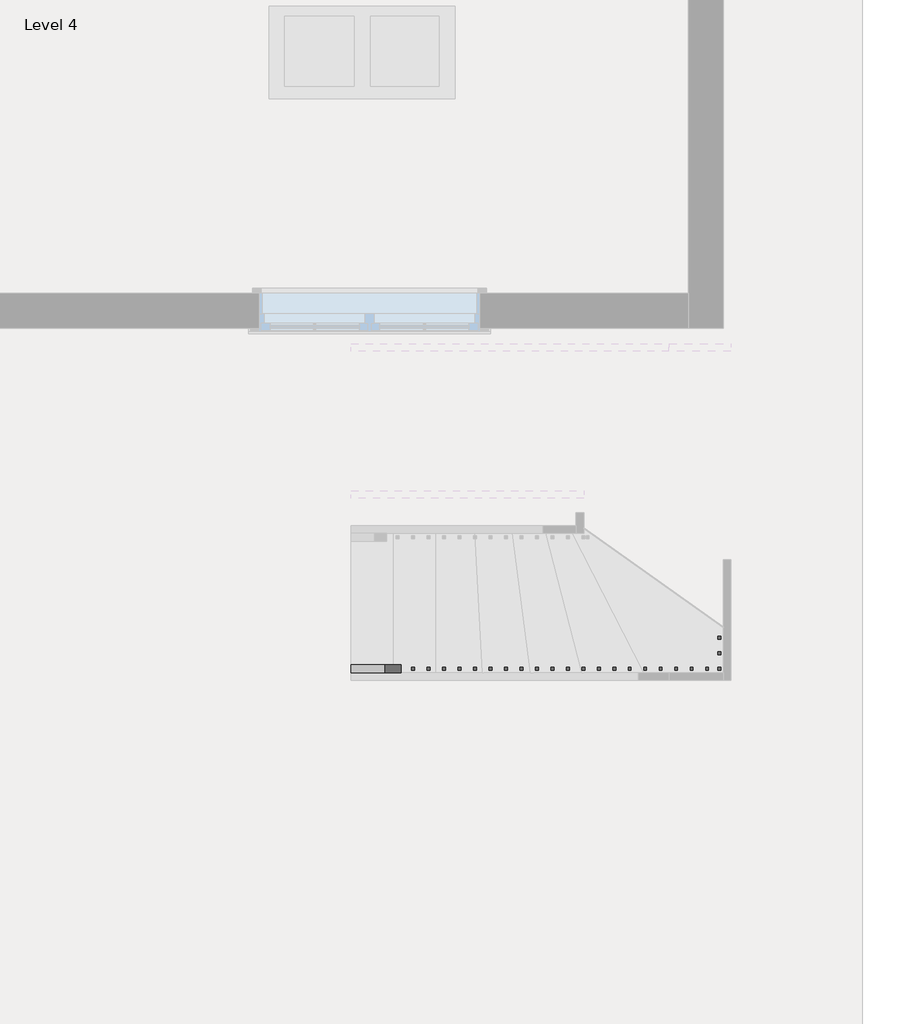
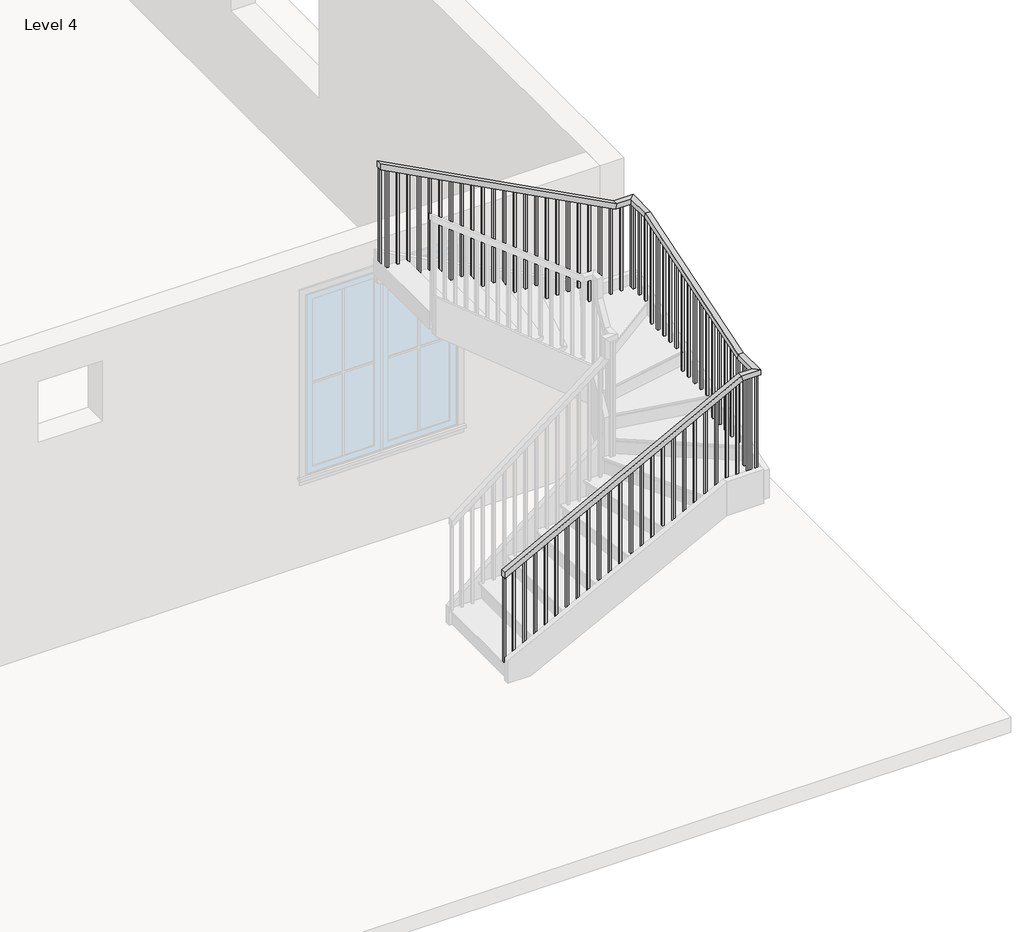
# One storey, part 2 of 3: 1 railing.
"""IFC4 building model written with IfcOpenShell, lengths in millimetres."""

from ifc_helpers import new_model, si_unit, frame, origin, place, context, project, spatial, polyline, outline, extrude, faceted_brep, element, save

model = new_model("IFC4")

# Units and contexts
model_context = context("Model", 3, world=origin())
ifc_project = project(units=[si_unit("LENGTHUNIT", "METRE", prefix="MILLI")], contexts=[model_context])

# Site, building, storey
site = spatial("IfcSite", under=ifc_project)
building = spatial("IfcBuilding", under=site)
storey = spatial("IfcBuildingStorey", under=building, Name="Level 4", Elevation=6400.8)

# Railing
placement = place(None, origin())
element("IfcRailing", 1, ObjectType="Handrail - Rectangular", at=placement, inside=storey, context=model_context, shape_type="SolidModel", body=[
    faceted_brep([(531.7538115, -7514.4090409, 7484.5333333), (531.7538115, -7514.4090409, 7427.0742652), (531.7538115, -7565.2090409, 7427.0742652), (531.7538115, -7565.2090409, 7484.5333333), (2789.4788736, -7514.4090409, 8677.8239201), (2802.0779381, -7514.4090409, 8627.0239201), (2802.0779381, -7565.2090409, 8627.0239201), (2789.4788736, -7565.2090409, 8677.8239201), (2923.0855034, -7269.9465826, 8627.0239201), (2923.0855034, -7277.8971587, 8677.8239201), (2923.0855034, -5744.320923, 9169.9094132), (2923.0855034, -5736.3703469, 9119.1094132), (2973.8855034, -7269.9465826, 8627.0239201), (2973.8855034, -5736.3703469, 9119.1094132), (2973.8855034, -7277.8971587, 8677.8239201), (2973.8855034, -5744.320923, 9169.9094132), (531.7538115, -5507.8090409, 10363.2), (531.7538115, -5457.0090409, 10363.2), (531.7538115, -5457.0090409, 10305.7409318), (531.7538115, -5507.8090409, 10305.7409318), (2776.879809, -5507.8090409, 9119.1094132), (2789.4788736, -5507.8090409, 9169.9094132), (2776.879809, -5457.0090409, 9119.1094132), (2789.4788736, -5457.0090409, 9169.9094132), (2923.0855034, -7514.4090409, 8677.8239201), (2923.0855034, -7514.4090409, 8627.0239201), (2973.8855034, -7565.2090409, 8627.0239201), (2973.8855034, -7565.2090409, 8677.8239201), (2923.0855034, -5507.8090409, 9169.9094132), (2923.0855034, -5507.8090409, 9119.1094132), (2973.8855034, -5457.0090409, 9119.1094132), (2973.8855034, -5457.0090409, 9169.9094132)], [[[0, 1, 2, 3]], [[1, 0, 4, 5]], [[2, 1, 5, 6]], [[3, 2, 6, 7]], [[0, 3, 7, 4]], [[8, 9, 10, 11]], [[12, 8, 11, 13]], [[14, 12, 13, 15]], [[9, 14, 15, 10]], [[16, 17, 18, 19]], [[20, 21, 16, 19]], [[22, 20, 19, 18]], [[23, 22, 18, 17]], [[21, 23, 17, 16]], [[5, 4, 24, 25]], [[6, 5, 25, 26]], [[7, 6, 26, 27]], [[4, 7, 27, 24]], [[25, 24, 9, 8]], [[26, 25, 8, 12]], [[27, 26, 12, 14]], [[24, 27, 14, 9]], [[11, 10, 28, 29]], [[13, 11, 29, 30]], [[15, 13, 30, 31]], [[10, 15, 31, 28]], [[29, 28, 21, 20]], [[30, 29, 20, 22]], [[31, 30, 22, 23]], [[28, 31, 23, 21]]]),
    extrude(outline(polyline([(10258.4597858, 621.2105034), (10268.5284102, 602.1605034), (9279.4666667, 602.1605034), (9279.4666667, 621.2105034), (10258.4597858, 621.2105034)])), frame((0.0, -5491.9340409, 0.0), z_axis=(0.0, 1.0, 0.0), x_axis=(0.0, 0.0, 1.0)), (0.0, 0.0, 1.0), 19.05),
    extrude(outline(polyline([(10204.7604556, 722.8105034), (10214.82908, 703.7605034), (9279.4666667, 703.7605034), (9279.4666667, 722.8105034), (10204.7604556, 722.8105034)])), frame((0.0, -5491.9340409, 0.0), z_axis=(0.0, 1.0, 0.0), x_axis=(0.0, 0.0, 1.0)), (0.0, 0.0, 1.0), 19.05),
    extrude(outline(polyline([(10151.0611254, 824.4105034), (10161.1297498, 805.3605034), (9110.1333333, 805.3605034), (9110.1333333, 824.4105034), (10151.0611254, 824.4105034)])), frame((0.0, -5491.9340409, 0.0), z_axis=(0.0, 1.0, 0.0), x_axis=(0.0, 0.0, 1.0)), (0.0, 0.0, 1.0), 19.05),
    extrude(outline(polyline([(10097.3617952, 926.0105034), (10107.4304196, 906.9605034), (9110.1333333, 906.9605034), (9110.1333333, 926.0105034), (10097.3617952, 926.0105034)])), frame((0.0, -5491.9340409, 0.0), z_axis=(0.0, 1.0, 0.0), x_axis=(0.0, 0.0, 1.0)), (0.0, 0.0, 1.0), 19.05),
    extrude(outline(polyline([(10043.662465, 1027.6105034), (10053.7310894, 1008.5605034), (9110.1333333, 1008.5605034), (9110.1333333, 1027.6105034), (10043.662465, 1027.6105034)])), frame((0.0, -5491.9340409, 0.0), z_axis=(0.0, 1.0, 0.0), x_axis=(0.0, 0.0, 1.0)), (0.0, 0.0, 1.0), 19.05),
    extrude(outline(polyline([(9989.9631348, 1129.2105034), (10000.0317592, 1110.1605034), (8940.8, 1110.1605034), (8940.8, 1129.2105034), (9989.9631348, 1129.2105034)])), frame((0.0, -5491.9340409, 0.0), z_axis=(0.0, 1.0, 0.0), x_axis=(0.0, 0.0, 1.0)), (0.0, 0.0, 1.0), 19.05),
    extrude(outline(polyline([(9936.2638046, 1230.8105034), (9946.332429, 1211.7605034), (8940.8, 1211.7605034), (8940.8, 1230.8105034), (9936.2638046, 1230.8105034)])), frame((0.0, -5491.9340409, 0.0), z_axis=(0.0, 1.0, 0.0), x_axis=(0.0, 0.0, 1.0)), (0.0, 0.0, 1.0), 19.05),
    extrude(outline(polyline([(9882.5644744, 1332.4105034), (9892.6330988, 1313.3605034), (8940.8, 1313.3605034), (8940.8, 1332.4105034), (9882.5644744, 1332.4105034)])), frame((0.0, -5491.9340409, 0.0), z_axis=(0.0, 1.0, 0.0), x_axis=(0.0, 0.0, 1.0)), (0.0, 0.0, 1.0), 19.05),
    extrude(outline(polyline([(9828.8651442, 1434.0105034), (9838.9337686, 1414.9605034), (8771.4666667, 1414.9605034), (8771.4666667, 1434.0105034), (9828.8651442, 1434.0105034)])), frame((0.0, -5491.9340409, 0.0), z_axis=(0.0, 1.0, 0.0), x_axis=(0.0, 0.0, 1.0)), (0.0, 0.0, 1.0), 19.05),
    extrude(outline(polyline([(9775.165814, 1535.6105034), (9785.2344384, 1516.5605034), (8771.4666667, 1516.5605034), (8771.4666667, 1535.6105034), (9775.165814, 1535.6105034)])), frame((0.0, -5491.9340409, 0.0), z_axis=(0.0, 1.0, 0.0), x_axis=(0.0, 0.0, 1.0)), (0.0, 0.0, 1.0), 19.05),
    extrude(outline(polyline([(9721.4664838, 1637.2105034), (9731.5351082, 1618.1605034), (8771.4666667, 1618.1605034), (8771.4666667, 1637.2105034), (9721.4664838, 1637.2105034)])), frame((0.0, -5491.9340409, 0.0), z_axis=(0.0, 1.0, 0.0), x_axis=(0.0, 0.0, 1.0)), (0.0, 0.0, 1.0), 19.05),
    extrude(outline(polyline([(9667.7671536, 1738.8105034), (9677.835778, 1719.7605034), (8602.1333333, 1719.7605034), (8602.1333333, 1738.8105034), (9667.7671536, 1738.8105034)])), frame((0.0, -5491.9340409, 0.0), z_axis=(0.0, 1.0, 0.0), x_axis=(0.0, 0.0, 1.0)), (0.0, 0.0, 1.0), 19.05),
    extrude(outline(polyline([(9614.0678234, 1840.4105034), (9624.1364478, 1821.3605034), (8602.1333333, 1821.3605034), (8602.1333333, 1840.4105034), (9614.0678234, 1840.4105034)])), frame((0.0, -5491.9340409, 0.0), z_axis=(0.0, 1.0, 0.0), x_axis=(0.0, 0.0, 1.0)), (0.0, 0.0, 1.0), 19.05),
    extrude(outline(polyline([(9560.3684932, 1942.0105034), (9570.4371176, 1922.9605034), (8602.1333333, 1922.9605034), (8602.1333333, 1942.0105034), (9560.3684932, 1942.0105034)])), frame((0.0, -5491.9340409, 0.0), z_axis=(0.0, 1.0, 0.0), x_axis=(0.0, 0.0, 1.0)), (0.0, 0.0, 1.0), 19.05),
    extrude(outline(polyline([(9506.669163, 2043.6105034), (9516.7377874, 2024.5605034), (8602.1333333, 2024.5605034), (8602.1333333, 2043.6105034), (9506.669163, 2043.6105034)])), frame((0.0, -5491.9340409, 0.0), z_axis=(0.0, 1.0, 0.0), x_axis=(0.0, 0.0, 1.0)), (0.0, 0.0, 1.0), 19.05),
    extrude(outline(polyline([(9452.9698328, 2145.2105034), (9463.0384572, 2126.1605034), (8432.8, 2126.1605034), (8432.8, 2145.2105034), (9452.9698328, 2145.2105034)])), frame((0.0, -5491.9340409, 0.0), z_axis=(0.0, 1.0, 0.0), x_axis=(0.0, 0.0, 1.0)), (0.0, 0.0, 1.0), 19.05),
    extrude(outline(polyline([(9399.2705026, 2246.8105034), (9409.339127, 2227.7605034), (8432.8, 2227.7605034), (8432.8, 2246.8105034), (9399.2705026, 2246.8105034)])), frame((0.0, -5491.9340409, 0.0), z_axis=(0.0, 1.0, 0.0), x_axis=(0.0, 0.0, 1.0)), (0.0, 0.0, 1.0), 19.05),
    extrude(outline(polyline([(9345.5711724, 2348.4105034), (9355.6397968, 2329.3605034), (8432.8, 2329.3605034), (8432.8, 2348.4105034), (9345.5711724, 2348.4105034)])), frame((0.0, -5491.9340409, 0.0), z_axis=(0.0, 1.0, 0.0), x_axis=(0.0, 0.0, 1.0)), (0.0, 0.0, 1.0), 19.05),
    extrude(outline(polyline([(9291.8718422, 2450.0105034), (9301.9404666, 2430.9605034), (8432.8, 2430.9605034), (8432.8, 2450.0105034), (9291.8718422, 2450.0105034)])), frame((0.0, -5491.9340409, 0.0), z_axis=(0.0, 1.0, 0.0), x_axis=(0.0, 0.0, 1.0)), (0.0, 0.0, 1.0), 19.05),
    extrude(outline(polyline([(9238.172512, 2551.6105034), (9248.2411364, 2532.5605034), (8263.4666667, 2532.5605034), (8263.4666667, 2551.6105034), (9238.172512, 2551.6105034)])), frame((0.0, -5491.9340409, 0.0), z_axis=(0.0, 1.0, 0.0), x_axis=(0.0, 0.0, 1.0)), (0.0, 0.0, 1.0), 19.05),
    extrude(outline(polyline([(9184.4731818, 2653.2105034), (9194.5418062, 2634.1605034), (8263.4666667, 2634.1605034), (8263.4666667, 2653.2105034), (9184.4731818, 2653.2105034)])), frame((0.0, -5491.9340409, 0.0), z_axis=(0.0, 1.0, 0.0), x_axis=(0.0, 0.0, 1.0)), (0.0, 0.0, 1.0), 19.05),
    extrude(outline(polyline([(9130.7738516, 2754.8105034), (9140.842476, 2735.7605034), (8263.4666667, 2735.7605034), (8263.4666667, 2754.8105034), (9130.7738516, 2754.8105034)])), frame((0.0, -5491.9340409, 0.0), z_axis=(0.0, 1.0, 0.0), x_axis=(0.0, 0.0, 1.0)), (0.0, 0.0, 1.0), 19.05),
    extrude(outline(polyline([(2856.4105034, -5472.8840409), (2856.4105034, -5491.9340409), (2837.3605034, -5491.9340409), (2837.3605034, -5472.8840409), (2856.4105034, -5472.8840409)])), frame((0.0, 0.0, 8263.4666667), z_axis=(0.0, 0.0, 1.0), x_axis=(1.0, 0.0, 0.0)), (0.0, 0.0, 1.0), 855.6427466),
    extrude(outline(polyline([(2958.0105034, -5517.3340409), (2938.9605034, -5517.3340409), (2938.9605034, -5498.2840409), (2958.0105034, -5498.2840409), (2958.0105034, -5517.3340409)])), frame((0.0, 0.0, 8263.4666667), z_axis=(0.0, 0.0, 1.0), x_axis=(1.0, 0.0, 0.0)), (0.0, 0.0, 1.0), 855.6427466),
    extrude(outline(polyline([(2958.0105034, -5618.9340409), (2938.9605034, -5618.9340409), (2938.9605034, -5599.8840409), (2958.0105034, -5599.8840409), (2958.0105034, -5618.9340409)])), frame((0.0, 0.0, 8263.4666667), z_axis=(0.0, 0.0, 1.0), x_axis=(1.0, 0.0, 0.0)), (0.0, 0.0, 1.0), 855.6427466),
    extrude(outline(polyline([(2958.0105034, -5720.5340409), (2938.9605034, -5720.5340409), (2938.9605034, -5701.4840409), (2958.0105034, -5701.4840409), (2958.0105034, -5720.5340409)])), frame((0.0, 0.0, 8263.4666667), z_axis=(0.0, 0.0, 1.0), x_axis=(1.0, 0.0, 0.0)), (0.0, 0.0, 1.0), 855.6427466),
    extrude(outline(polyline([(-5822.1340409, 9091.5900316), (-5803.0840409, 9097.7026907), (-5803.0840409, 8094.1333333), (-5822.1340409, 8094.1333333), (-5822.1340409, 9091.5900316)])), frame((2938.9605034, 0.0, 0.0), z_axis=(1.0, 0.0, 0.0), x_axis=(0.0, 1.0, 0.0)), (0.0, 0.0, 1.0), 19.05),
    extrude(outline(polyline([(-5923.7340409, 9058.9891834), (-5904.6840409, 9065.1018425), (-5904.6840409, 8094.1333333), (-5923.7340409, 8094.1333333), (-5923.7340409, 9058.9891834)])), frame((2938.9605034, 0.0, 0.0), z_axis=(1.0, 0.0, 0.0), x_axis=(0.0, 1.0, 0.0)), (0.0, 0.0, 1.0), 19.05),
    extrude(outline(polyline([(-6025.3340409, 9026.3883352), (-6006.2840409, 9032.5009942), (-6006.2840409, 8094.1333333), (-6025.3340409, 8094.1333333), (-6025.3340409, 9026.3883352)])), frame((2938.9605034, 0.0, 0.0), z_axis=(1.0, 0.0, 0.0), x_axis=(0.0, 1.0, 0.0)), (0.0, 0.0, 1.0), 19.05),
    extrude(outline(polyline([(-6126.9340409, 8993.787487), (-6107.8840409, 8999.900146), (-6107.8840409, 8094.1333333), (-6126.9340409, 8094.1333333), (-6126.9340409, 8993.787487)])), frame((2938.9605034, 0.0, 0.0), z_axis=(1.0, 0.0, 0.0), x_axis=(0.0, 1.0, 0.0)), (0.0, 0.0, 1.0), 19.05),
    extrude(outline(polyline([(-6228.5340409, 8961.1866387), (-6209.4840409, 8967.2992978), (-6209.4840409, 8094.1333333), (-6228.5340409, 8094.1333333), (-6228.5340409, 8961.1866387)])), frame((2938.9605034, 0.0, 0.0), z_axis=(1.0, 0.0, 0.0), x_axis=(0.0, 1.0, 0.0)), (0.0, 0.0, 1.0), 19.05),
    extrude(outline(polyline([(-6330.1340409, 8928.5857905), (-6311.0840409, 8934.6984495), (-6311.0840409, 7924.8), (-6330.1340409, 7924.8), (-6330.1340409, 8928.5857905)])), frame((2938.9605034, 0.0, 0.0), z_axis=(1.0, 0.0, 0.0), x_axis=(0.0, 1.0, 0.0)), (0.0, 0.0, 1.0), 19.05),
    extrude(outline(polyline([(-6431.7340409, 8895.9849423), (-6412.6840409, 8902.0976013), (-6412.6840409, 7924.8), (-6431.7340409, 7924.8), (-6431.7340409, 8895.9849423)])), frame((2938.9605034, 0.0, 0.0), z_axis=(1.0, 0.0, 0.0), x_axis=(0.0, 1.0, 0.0)), (0.0, 0.0, 1.0), 19.05),
    extrude(outline(polyline([(-6533.3340409, 8863.384094), (-6514.2840409, 8869.4967531), (-6514.2840409, 7924.8), (-6533.3340409, 7924.8), (-6533.3340409, 8863.384094)])), frame((2938.9605034, 0.0, 0.0), z_axis=(1.0, 0.0, 0.0), x_axis=(0.0, 1.0, 0.0)), (0.0, 0.0, 1.0), 19.05),
    extrude(outline(polyline([(-6634.9340409, 8830.7832458), (-6615.8840409, 8836.8959049), (-6615.8840409, 7924.8), (-6634.9340409, 7924.8), (-6634.9340409, 8830.7832458)])), frame((2938.9605034, 0.0, 0.0), z_axis=(1.0, 0.0, 0.0), x_axis=(0.0, 1.0, 0.0)), (0.0, 0.0, 1.0), 19.05),
    extrude(outline(polyline([(-6736.5340409, 8798.1823976), (-6717.4840409, 8804.2950566), (-6717.4840409, 7924.8), (-6736.5340409, 7924.8), (-6736.5340409, 8798.1823976)])), frame((2938.9605034, 0.0, 0.0), z_axis=(1.0, 0.0, 0.0), x_axis=(0.0, 1.0, 0.0)), (0.0, 0.0, 1.0), 19.05),
    extrude(outline(polyline([(-6838.1340409, 8765.5815494), (-6819.0840409, 8771.6942084), (-6819.0840409, 7755.4666667), (-6838.1340409, 7755.4666667), (-6838.1340409, 8765.5815494)])), frame((2938.9605034, 0.0, 0.0), z_axis=(1.0, 0.0, 0.0), x_axis=(0.0, 1.0, 0.0)), (0.0, 0.0, 1.0), 19.05),
    extrude(outline(polyline([(-6939.7340409, 8732.9807011), (-6920.6840409, 8739.0933602), (-6920.6840409, 7755.4666667), (-6939.7340409, 7755.4666667), (-6939.7340409, 8732.9807011)])), frame((2938.9605034, 0.0, 0.0), z_axis=(1.0, 0.0, 0.0), x_axis=(0.0, 1.0, 0.0)), (0.0, 0.0, 1.0), 19.05),
    extrude(outline(polyline([(-7041.3340409, 8700.3798529), (-7022.2840409, 8706.492512), (-7022.2840409, 7755.4666667), (-7041.3340409, 7755.4666667), (-7041.3340409, 8700.3798529)])), frame((2938.9605034, 0.0, 0.0), z_axis=(1.0, 0.0, 0.0), x_axis=(0.0, 1.0, 0.0)), (0.0, 0.0, 1.0), 19.05),
    extrude(outline(polyline([(-7142.9340409, 8667.7790047), (-7123.8840409, 8673.8916637), (-7123.8840409, 7755.4666667), (-7142.9340409, 7755.4666667), (-7142.9340409, 8667.7790047)])), frame((2938.9605034, 0.0, 0.0), z_axis=(1.0, 0.0, 0.0), x_axis=(0.0, 1.0, 0.0)), (0.0, 0.0, 1.0), 19.05),
    extrude(outline(polyline([(-7244.5340409, 8635.1781565), (-7225.4840409, 8641.2908155), (-7225.4840409, 7755.4666667), (-7244.5340409, 7755.4666667), (-7244.5340409, 8635.1781565)])), frame((2938.9605034, 0.0, 0.0), z_axis=(1.0, 0.0, 0.0), x_axis=(0.0, 1.0, 0.0)), (0.0, 0.0, 1.0), 19.05),
    extrude(outline(polyline([(2958.0105034, -7346.1340409), (2938.9605034, -7346.1340409), (2938.9605034, -7327.0840409), (2958.0105034, -7327.0840409), (2958.0105034, -7346.1340409)])), frame((0.0, 0.0, 7586.1333333), z_axis=(0.0, 0.0, 1.0), x_axis=(1.0, 0.0, 0.0)), (0.0, 0.0, 1.0), 1040.8905868),
    extrude(outline(polyline([(2958.0105034, -7447.7340409), (2938.9605034, -7447.7340409), (2938.9605034, -7428.6840409), (2958.0105034, -7428.6840409), (2958.0105034, -7447.7340409)])), frame((0.0, 0.0, 7586.1333333), z_axis=(0.0, 0.0, 1.0), x_axis=(1.0, 0.0, 0.0)), (0.0, 0.0, 1.0), 1040.8905868),
    extrude(outline(polyline([(2859.0288115, -7549.3340409), (2859.0288115, -7530.2840409), (2878.0788115, -7530.2840409), (2878.0788115, -7549.3340409), (2859.0288115, -7549.3340409)])), frame((0.0, 0.0, 7586.1333333), z_axis=(0.0, 0.0, 1.0), x_axis=(1.0, 0.0, 0.0)), (0.0, 0.0, 1.0), 1040.8905868),
    extrude(outline(polyline([(8613.4938418, 2776.4788115), (8603.4252174, 2757.4288115), (7586.1333333, 2757.4288115), (7586.1333333, 2776.4788115), (8613.4938418, 2776.4788115)])), frame((0.0, -7549.3340409, 0.0), z_axis=(0.0, 1.0, 0.0), x_axis=(0.0, 0.0, 1.0)), (0.0, 0.0, 1.0), 19.05),
    extrude(outline(polyline([(8559.7945116, 2674.8788115), (8549.7258872, 2655.8288115), (7586.1333333, 2655.8288115), (7586.1333333, 2674.8788115), (8559.7945116, 2674.8788115)])), frame((0.0, -7549.3340409, 0.0), z_axis=(0.0, 1.0, 0.0), x_axis=(0.0, 0.0, 1.0)), (0.0, 0.0, 1.0), 19.05),
    extrude(outline(polyline([(8506.0951814, 2573.2788115), (8496.026557, 2554.2288115), (7586.1333333, 2554.2288115), (7586.1333333, 2573.2788115), (8506.0951814, 2573.2788115)])), frame((0.0, -7549.3340409, 0.0), z_axis=(0.0, 1.0, 0.0), x_axis=(0.0, 0.0, 1.0)), (0.0, 0.0, 1.0), 19.05),
    extrude(outline(polyline([(8452.3958512, 2471.6788115), (8442.3272268, 2452.6288115), (7586.1333333, 2452.6288115), (7586.1333333, 2471.6788115), (8452.3958512, 2471.6788115)])), frame((0.0, -7549.3340409, 0.0), z_axis=(0.0, 1.0, 0.0), x_axis=(0.0, 0.0, 1.0)), (0.0, 0.0, 1.0), 19.05),
    extrude(outline(polyline([(8398.696521, 2370.0788115), (8388.6278966, 2351.0288115), (7416.8, 2351.0288115), (7416.8, 2370.0788115), (8398.696521, 2370.0788115)])), frame((0.0, -7549.3340409, 0.0), z_axis=(0.0, 1.0, 0.0), x_axis=(0.0, 0.0, 1.0)), (0.0, 0.0, 1.0), 19.05),
    extrude(outline(polyline([(8344.9971908, 2268.4788115), (8334.9285664, 2249.4288115), (7416.8, 2249.4288115), (7416.8, 2268.4788115), (8344.9971908, 2268.4788115)])), frame((0.0, -7549.3340409, 0.0), z_axis=(0.0, 1.0, 0.0), x_axis=(0.0, 0.0, 1.0)), (0.0, 0.0, 1.0), 19.05),
    extrude(outline(polyline([(8291.2978606, 2166.8788115), (8281.2292362, 2147.8288115), (7416.8, 2147.8288115), (7416.8, 2166.8788115), (8291.2978606, 2166.8788115)])), frame((0.0, -7549.3340409, 0.0), z_axis=(0.0, 1.0, 0.0), x_axis=(0.0, 0.0, 1.0)), (0.0, 0.0, 1.0), 19.05),
    extrude(outline(polyline([(8237.5985304, 2065.2788115), (8227.529906, 2046.2288115), (7416.8, 2046.2288115), (7416.8, 2065.2788115), (8237.5985304, 2065.2788115)])), frame((0.0, -7549.3340409, 0.0), z_axis=(0.0, 1.0, 0.0), x_axis=(0.0, 0.0, 1.0)), (0.0, 0.0, 1.0), 19.05),
    extrude(outline(polyline([(8183.8992002, 1963.6788115), (8173.8305758, 1944.6288115), (7247.4666667, 1944.6288115), (7247.4666667, 1963.6788115), (8183.8992002, 1963.6788115)])), frame((0.0, -7549.3340409, 0.0), z_axis=(0.0, 1.0, 0.0), x_axis=(0.0, 0.0, 1.0)), (0.0, 0.0, 1.0), 19.05),
    extrude(outline(polyline([(8130.19987, 1862.0788115), (8120.1312456, 1843.0288115), (7247.4666667, 1843.0288115), (7247.4666667, 1862.0788115), (8130.19987, 1862.0788115)])), frame((0.0, -7549.3340409, 0.0), z_axis=(0.0, 1.0, 0.0), x_axis=(0.0, 0.0, 1.0)), (0.0, 0.0, 1.0), 19.05),
    extrude(outline(polyline([(8076.5005398, 1760.4788115), (8066.4319154, 1741.4288115), (7247.4666667, 1741.4288115), (7247.4666667, 1760.4788115), (8076.5005398, 1760.4788115)])), frame((0.0, -7549.3340409, 0.0), z_axis=(0.0, 1.0, 0.0), x_axis=(0.0, 0.0, 1.0)), (0.0, 0.0, 1.0), 19.05),
    extrude(outline(polyline([(8022.8012096, 1658.8788115), (8012.7325852, 1639.8288115), (7078.1333333, 1639.8288115), (7078.1333333, 1658.8788115), (8022.8012096, 1658.8788115)])), frame((0.0, -7549.3340409, 0.0), z_axis=(0.0, 1.0, 0.0), x_axis=(0.0, 0.0, 1.0)), (0.0, 0.0, 1.0), 19.05),
    extrude(outline(polyline([(7969.1018794, 1557.2788115), (7959.033255, 1538.2288115), (7078.1333333, 1538.2288115), (7078.1333333, 1557.2788115), (7969.1018794, 1557.2788115)])), frame((0.0, -7549.3340409, 0.0), z_axis=(0.0, 1.0, 0.0), x_axis=(0.0, 0.0, 1.0)), (0.0, 0.0, 1.0), 19.05),
    extrude(outline(polyline([(7915.4025492, 1455.6788115), (7905.3339248, 1436.6288115), (7078.1333333, 1436.6288115), (7078.1333333, 1455.6788115), (7915.4025492, 1455.6788115)])), frame((0.0, -7549.3340409, 0.0), z_axis=(0.0, 1.0, 0.0), x_axis=(0.0, 0.0, 1.0)), (0.0, 0.0, 1.0), 19.05),
    extrude(outline(polyline([(7861.703219, 1354.0788115), (7851.6345946, 1335.0288115), (6908.8, 1335.0288115), (6908.8, 1354.0788115), (7861.703219, 1354.0788115)])), frame((0.0, -7549.3340409, 0.0), z_axis=(0.0, 1.0, 0.0), x_axis=(0.0, 0.0, 1.0)), (0.0, 0.0, 1.0), 19.05),
    extrude(outline(polyline([(7808.0038888, 1252.4788115), (7797.9352644, 1233.4288115), (6908.8, 1233.4288115), (6908.8, 1252.4788115), (7808.0038888, 1252.4788115)])), frame((0.0, -7549.3340409, 0.0), z_axis=(0.0, 1.0, 0.0), x_axis=(0.0, 0.0, 1.0)), (0.0, 0.0, 1.0), 19.05),
    extrude(outline(polyline([(7754.3045586, 1150.8788115), (7744.2359342, 1131.8288115), (6908.8, 1131.8288115), (6908.8, 1150.8788115), (7754.3045586, 1150.8788115)])), frame((0.0, -7549.3340409, 0.0), z_axis=(0.0, 1.0, 0.0), x_axis=(0.0, 0.0, 1.0)), (0.0, 0.0, 1.0), 19.05),
    extrude(outline(polyline([(7700.6052284, 1049.2788115), (7690.536604, 1030.2288115), (6739.4666667, 1030.2288115), (6739.4666667, 1049.2788115), (7700.6052284, 1049.2788115)])), frame((0.0, -7549.3340409, 0.0), z_axis=(0.0, 1.0, 0.0), x_axis=(0.0, 0.0, 1.0)), (0.0, 0.0, 1.0), 19.05),
    extrude(outline(polyline([(7646.9058982, 947.6788115), (7636.8372738, 928.6288115), (6739.4666667, 928.6288115), (6739.4666667, 947.6788115), (7646.9058982, 947.6788115)])), frame((0.0, -7549.3340409, 0.0), z_axis=(0.0, 1.0, 0.0), x_axis=(0.0, 0.0, 1.0)), (0.0, 0.0, 1.0), 19.05),
    extrude(outline(polyline([(7593.206568, 846.0788115), (7583.1379436, 827.0288115), (6739.4666667, 827.0288115), (6739.4666667, 846.0788115), (7593.206568, 846.0788115)])), frame((0.0, -7549.3340409, 0.0), z_axis=(0.0, 1.0, 0.0), x_axis=(0.0, 0.0, 1.0)), (0.0, 0.0, 1.0), 19.05),
    extrude(outline(polyline([(7539.5072378, 744.4788115), (7529.4386134, 725.4288115), (6570.1333333, 725.4288115), (6570.1333333, 744.4788115), (7539.5072378, 744.4788115)])), frame((0.0, -7549.3340409, 0.0), z_axis=(0.0, 1.0, 0.0), x_axis=(0.0, 0.0, 1.0)), (0.0, 0.0, 1.0), 19.05),
    extrude(outline(polyline([(7485.8079076, 642.8788115), (7475.7392831, 623.8288115), (6570.1333333, 623.8288115), (6570.1333333, 642.8788115), (7485.8079076, 642.8788115)])), frame((0.0, -7549.3340409, 0.0), z_axis=(0.0, 1.0, 0.0), x_axis=(0.0, 0.0, 1.0)), (0.0, 0.0, 1.0), 19.05),
    extrude(outline(polyline([(2958.0105034, -5491.9340409), (2938.9605034, -5491.9340409), (2938.9605034, -5472.8840409), (2958.0105034, -5472.8840409), (2958.0105034, -5491.9340409)])), frame((0.0, 0.0, 8263.4666667), z_axis=(0.0, 0.0, 1.0), x_axis=(1.0, 0.0, 0.0)), (0.0, 0.0, 1.0), 855.6427466),
    extrude(outline(polyline([(2938.9605034, -7549.3340409), (2938.9605034, -7530.2840409), (2958.0105034, -7530.2840409), (2958.0105034, -7549.3340409), (2938.9605034, -7549.3340409)])), frame((0.0, 0.0, 7586.1333333), z_axis=(0.0, 0.0, 1.0), x_axis=(1.0, 0.0, 0.0)), (0.0, 0.0, 1.0), 1040.8905868),
    extrude(outline(polyline([(10295.6723074, 550.8038115), (10305.7409318, 531.7538115), (9279.4666667, 531.7538115), (9279.4666667, 550.8038115), (10295.6723074, 550.8038115)])), frame((0.0, -5491.9340409, 0.0), z_axis=(0.0, 1.0, 0.0), x_axis=(0.0, 0.0, 1.0)), (0.0, 0.0, 1.0), 19.05),
    extrude(outline(polyline([(7437.1428896, 550.8038115), (7427.0742652, 531.7538115), (6570.1333333, 531.7538115), (6570.1333333, 550.8038115), (7437.1428896, 550.8038115)])), frame((0.0, -7549.3340409, 0.0), z_axis=(0.0, 1.0, 0.0), x_axis=(0.0, 0.0, 1.0)), (0.0, 0.0, 1.0), 19.05),
])

save(model, "model.ifc")

# Revit data of these elements
# Type "Handrail - Rectangular"
#   Assembly Code = "C2010400"
#   built-in parameter 1008612 = 0.0416667 (stored number, unit not read)
#   built-in parameter 1008611 = 0.0416667 (stored number, unit not read)
#   built-in parameter 1008609 = 0.333333 (stored number, unit not read)
#   built-in parameter 1008604 = 0.166667 (stored number, unit not read)
#   built-in parameter 1008603 = 0.166667 (stored number, unit not read)
#   Railing Height = 3' - 0"
#   built-in parameter 1008630 = 2
#   built-in parameter 1008610 = 2
#   built-in parameter 1008618 = Baluster - Square : 3/4"
# Element 1 (IfcRailing, "Handrail - Rectangular")
#   Phase Created = New Construction
